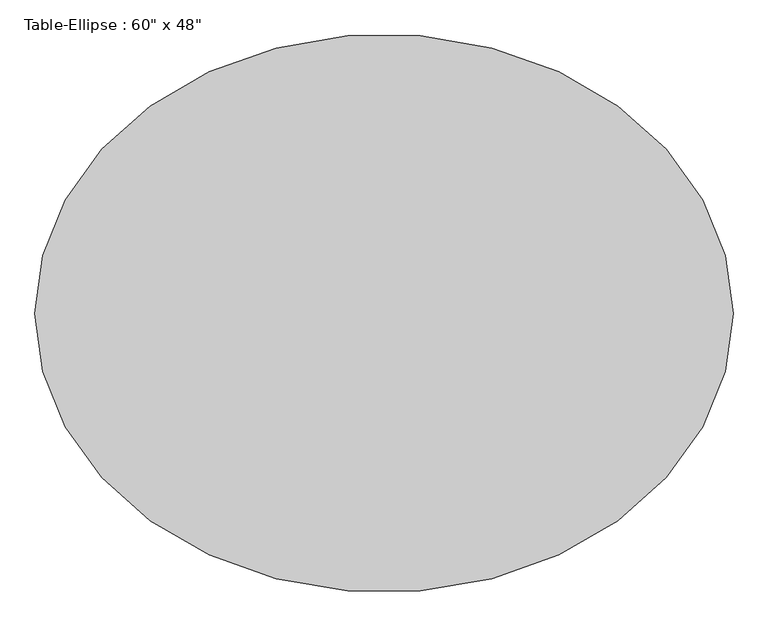
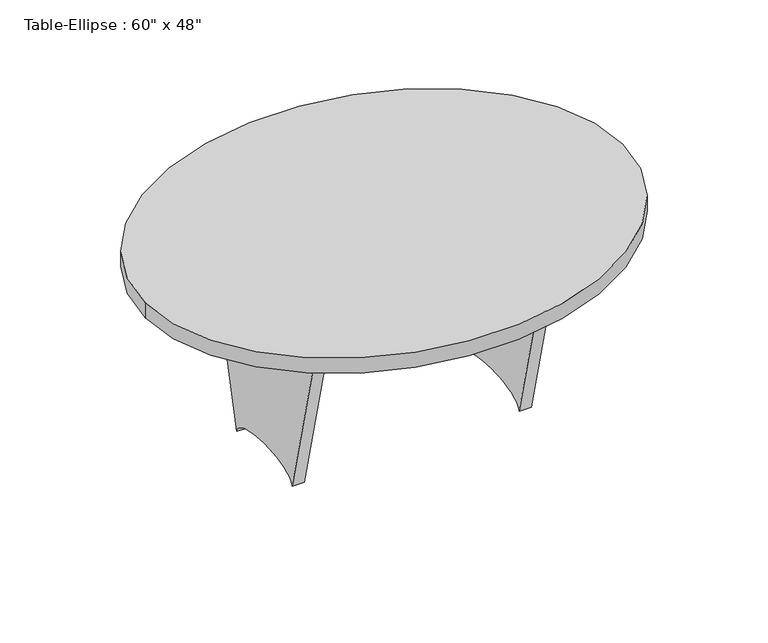
"""IFC4 building model written with IfcOpenShell, lengths in millimetres: furniture geometry."""

from ifc_helpers import new_model, si_unit, point, frame, origin, place, context, project, spatial, ellipse_curve, trimmed, source, transform, mapped, element, save
from ifc_brep_helpers import plane_surface, extruded_surface, advanced_brep


def furniture_ad1c254c(model_context):
    return source(origin(), model_context, "Body", "AdvancedBrep", [
        advanced_brep(
        [(-342.9, 19.05, 609.6), (342.9, 19.05, 609.6), (342.9, 19.05, 406.4), (-342.9, 19.05, 406.4), (-342.9, -19.05, 609.6), (-342.9, -19.05, 406.4), (342.9, -19.05, 406.4), (342.9, -19.05, 609.6)],
        [
            (0, 1),
            (1, 2),
            (2, 3, ellipse_curve(frame((0.0, 19.05, 406.4), z_axis=(0.0, -1.0, 0.0), x_axis=(1.0, 0.0, 0.0)), 342.9, 101.6)),
            (3, 0),
            (4, 5),
            (5, 6, ellipse_curve(frame((0.0, -19.05, 406.4), z_axis=(0.0, 1.0, 0.0), x_axis=(1.0, 0.0, 0.0)), 342.9, 101.6)),
            (6, 7),
            (7, 4),
            (0, 4),
            (7, 1),
            (6, 2),
            (5, 3),
        ],
        [
            plane_surface(frame((-342.9, 19.05, 609.6), z_axis=(0.0, 1.0, 0.0), x_axis=(1.0, 0.0, 0.0))),
            plane_surface(frame((-342.9, -19.05, 609.6), z_axis=(0.0, -1.0, 0.0), x_axis=(-1.0, 0.0, 0.0))),
            plane_surface(frame((-342.9, 19.05, 609.6), z_axis=(0.0, 0.0, 1.0), x_axis=(0.0, -1.0, 0.0))),
            plane_surface(frame((342.9, 19.05, 609.6), z_axis=(1.0, 0.0, 0.0), x_axis=(0.0, -1.0, 0.0))),
            extruded_surface(trimmed(ellipse_curve(frame((0.0, -57.15, 406.4), z_axis=(0.0, -1.0, 0.0), x_axis=(1.0, 0.0, 0.0)), 342.9, 101.6), [point((342.9, -57.15, 406.4))], [point((-342.9, -57.15, 406.4))], True, "CARTESIAN"), (0.0, 38.099999999999994, 0.0), 38.099999999999994),
            plane_surface(frame((-342.9, 19.05, 406.4), z_axis=(-1.0, 0.0, 0.0), x_axis=(0.0, -1.0, 0.0))),
        ],
        [
            (0, [[1, 2, 3, 4]]),
            (1, [[5, 6, 7, 8]]),
            (2, [[-1, 9, -8, 10]]),
            (3, [[-2, -10, -7, 11]]),
            (4, [[-3, -11, -6, 12]]),
            (5, [[-4, -12, -5, -9]]),
        ],
    ),
        advanced_brep(
        [(381.0, 304.8, 609.6), (381.0, -304.8, 609.6), (381.0, -152.4, 0.0), (381.0, 152.4, 0.0), (342.9, 304.8, 609.6), (342.9, 152.4, 0.0), (342.9, -152.4, 0.0), (342.9, -304.8, 609.6)],
        [
            (0, 1),
            (1, 2),
            (2, 3, ellipse_curve(frame((381.0, 0.0, 0.0), z_axis=(-1.0, 0.0, 0.0), x_axis=(0.0, 1.0, 0.0)), 152.4, 50.8)),
            (3, 0),
            (4, 5),
            (5, 6, ellipse_curve(frame((342.9, 0.0, 0.0), z_axis=(1.0, 0.0, 0.0), x_axis=(0.0, 1.0, 0.0)), 152.4, 50.8)),
            (6, 7),
            (7, 4),
            (0, 4),
            (7, 1),
            (6, 2),
            (5, 3),
        ],
        [
            plane_surface(frame((381.0, -304.8, 609.6), z_axis=(1.0, 0.0, 0.0), x_axis=(0.0, -1.0, 0.0))),
            plane_surface(frame((342.9, -304.8, 609.6), z_axis=(-1.0, 0.0, 0.0), x_axis=(0.0, 1.0, 0.0))),
            plane_surface(frame((381.0, 304.8, 609.6), z_axis=(0.0, 0.0, 1.0), x_axis=(-1.0, 0.0, 0.0))),
            plane_surface(frame((381.0, -304.8, 609.6), z_axis=(0.0, -0.9701425001453307, -0.24253562503633866), x_axis=(-1.0, 0.0, 0.0))),
            extruded_surface(trimmed(ellipse_curve(frame((304.8, 0.0, 0.0), z_axis=(-1.0, 0.0, 0.0), x_axis=(0.0, 1.0, 0.0)), 152.4, 50.8), [point((304.8, -152.4, 0.0))], [point((304.8, 152.4, 0.0))], True, "CARTESIAN"), (38.099999999999966, 0.0, 0.0), 38.099999999999966),
            plane_surface(frame((381.0, 152.4, 0.0), z_axis=(0.0, 0.9701425001453345, -0.24253562503632273), x_axis=(-1.0, 0.0, 0.0))),
        ],
        [
            (0, [[1, 2, 3, 4]]),
            (1, [[5, 6, 7, 8]]),
            (2, [[-1, 9, -8, 10]]),
            (3, [[-2, -10, -7, 11]]),
            (4, [[-3, -11, -6, 12]]),
            (5, [[-4, -12, -5, -9]]),
        ],
    ),
        advanced_brep(
        [(-342.9, 304.8, 609.6), (-342.9, -304.8, 609.6), (-342.9, -152.4, 0.0), (-342.9, 152.4, 0.0), (-381.0, 304.8, 609.6), (-381.0, 152.4, 0.0), (-381.0, -152.4, 0.0), (-381.0, -304.8, 609.6)],
        [
            (0, 1),
            (1, 2),
            (2, 3, ellipse_curve(frame((-342.9, 0.0, 0.0), z_axis=(-1.0, 0.0, 0.0), x_axis=(0.0, 1.0, 0.0)), 152.4, 50.8)),
            (3, 0),
            (4, 5),
            (5, 6, ellipse_curve(frame((-381.0, 0.0, 0.0), z_axis=(1.0, 0.0, 0.0), x_axis=(0.0, 1.0, 0.0)), 152.4, 50.8)),
            (6, 7),
            (7, 4),
            (0, 4),
            (7, 1),
            (6, 2),
            (5, 3),
        ],
        [
            plane_surface(frame((-342.9, -304.8, 609.6), z_axis=(1.0, 0.0, 0.0), x_axis=(0.0, -1.0, 0.0))),
            plane_surface(frame((-381.0, -304.8, 609.6), z_axis=(-1.0, 0.0, 0.0), x_axis=(0.0, 1.0, 0.0))),
            plane_surface(frame((-342.9, 304.8, 609.6), z_axis=(0.0, 0.0, 1.0), x_axis=(-1.0, 0.0, 0.0))),
            plane_surface(frame((-342.9, -304.8, 609.6), z_axis=(0.0, -0.9701425001453302, -0.24253562503633994), x_axis=(-1.0, 0.0, 0.0))),
            extruded_surface(trimmed(ellipse_curve(frame((-419.1, 0.0, 0.0), z_axis=(-1.0, 0.0, 0.0), x_axis=(0.0, 1.0, 0.0)), 152.4, 50.8), [point((-419.1, -152.4, 0.0))], [point((-419.1, 152.4, 0.0))], True, "CARTESIAN"), (38.10000000000002, 0.0, 0.0), 38.10000000000002),
            plane_surface(frame((-342.9, 152.4, 0.0), z_axis=(0.0, 0.9701425001453328, -0.24253562503632956), x_axis=(-1.0, 0.0, 0.0))),
        ],
        [
            (0, [[1, 2, 3, 4]]),
            (1, [[5, 6, 7, 8]]),
            (2, [[-1, 9, -8, 10]]),
            (3, [[-2, -10, -7, 11]]),
            (4, [[-3, -11, -6, 12]]),
            (5, [[-4, -12, -5, -9]]),
        ],
    ),
        advanced_brep(
        [(-762.0, 0.0, 660.4), (762.0, 0.0, 660.4), (-762.0, 0.0, 609.6), (762.0, 0.0, 609.6)],
        [
            (0, 1, ellipse_curve(frame((0.0, 0.0, 660.4), z_axis=(0.0, 0.0, 1.0), x_axis=(1.0, 0.0, 0.0)), 762.0, 609.6)),
            (1, 0, ellipse_curve(frame((0.0, 0.0, 660.4), z_axis=(0.0, 0.0, 1.0), x_axis=(1.0, 0.0, 0.0)), 762.0, 609.6)),
            (2, 3, ellipse_curve(frame((0.0, 0.0, 609.6), z_axis=(0.0, 0.0, -1.0), x_axis=(1.0, 0.0, 0.0)), 762.0, 609.6)),
            (3, 2, ellipse_curve(frame((0.0, 0.0, 609.6), z_axis=(0.0, 0.0, -1.0), x_axis=(1.0, 0.0, 0.0)), 762.0, 609.6)),
            (0, 2),
            (3, 1),
        ],
        [
            plane_surface(frame((762.0, 0.0, 660.4), z_axis=(0.0, 0.0, 1.0), x_axis=(0.0, 1.0, 0.0))),
            plane_surface(frame((762.0, 0.0, 609.6), z_axis=(0.0, 0.0, -1.0), x_axis=(0.0, -1.0, 0.0))),
            extruded_surface(trimmed(ellipse_curve(frame((0.0, 0.0, 558.8), z_axis=(0.0, 0.0, 1.0), x_axis=(1.0, 0.0, 0.0)), 762.0, 609.6), [point((-762.0, 0.0, 558.8))], [point((762.0, 0.0, 558.8))], True, "CARTESIAN"), (0.0, 0.0, 50.80000000000007), 50.80000000000007),
            extruded_surface(trimmed(ellipse_curve(frame((0.0, 0.0, 558.8), z_axis=(0.0, 0.0, 1.0), x_axis=(1.0, 0.0, 0.0)), 762.0, 609.6), [point((762.0, 0.0, 558.8))], [point((-762.0, 0.0, 558.8))], True, "CARTESIAN"), (0.0, 0.0, 50.80000000000007), 50.80000000000007),
        ],
        [
            (0, [[1, 2]]),
            (1, [[3, 4]]),
            (2, [[-1, 5, -4, 6]]),
            (3, [[-2, -6, -3, -5]]),
        ],
    ),
    ])


if __name__ == "__main__":
    model = new_model("IFC4")
    model_context = context("Model", 3, world=origin())
    ifc_project = project(units=[si_unit("LENGTHUNIT", "METRE", prefix="MILLI")], contexts=[model_context])
    site = spatial("IfcSite", under=ifc_project)
    building = spatial("IfcBuilding", under=site)
    placement = place(None, origin())
    furniture_shape = furniture_ad1c254c(model_context)
    element("IfcFurniture", 1, ObjectType="Table-Ellipse : 60\" x 48\"", at=placement, inside=building, context=model_context, shape_type="MappedRepresentation", body=[
        mapped(furniture_shape, transform((0.0, 0.0, 0.0), x_axis=(1.0, 0.0, 0.0), y_axis=(0.0, 1.0, 0.0), z_axis=(0.0, 0.0, 1.0))),
    ])
    save(model, "model.ifc")

# Revit data of these elements
# Type "Table-Ellipse : 60\" x 48\""
#   Assembly Code = "E2020200"
#   Half Width = 2' - 0"
#   Half Length = 2' - 6"
#   Height = 2' - 2"
#   Length = 5' - 0"
#   Width = 4' - 0"
#   Base Material = Birch
#   Top Material = Birch
#   Default Elevation = 0
# Element 1 (IfcFurniture, "Table-Ellipse : 60\" x 48\"")
#   Materials on its faces: "Birch"
# Materials
#   "Birch": class "Wood", colour RGB 224 178 126, transparency 0, Description = "Betula Alleghaniensis", Cost = 0
